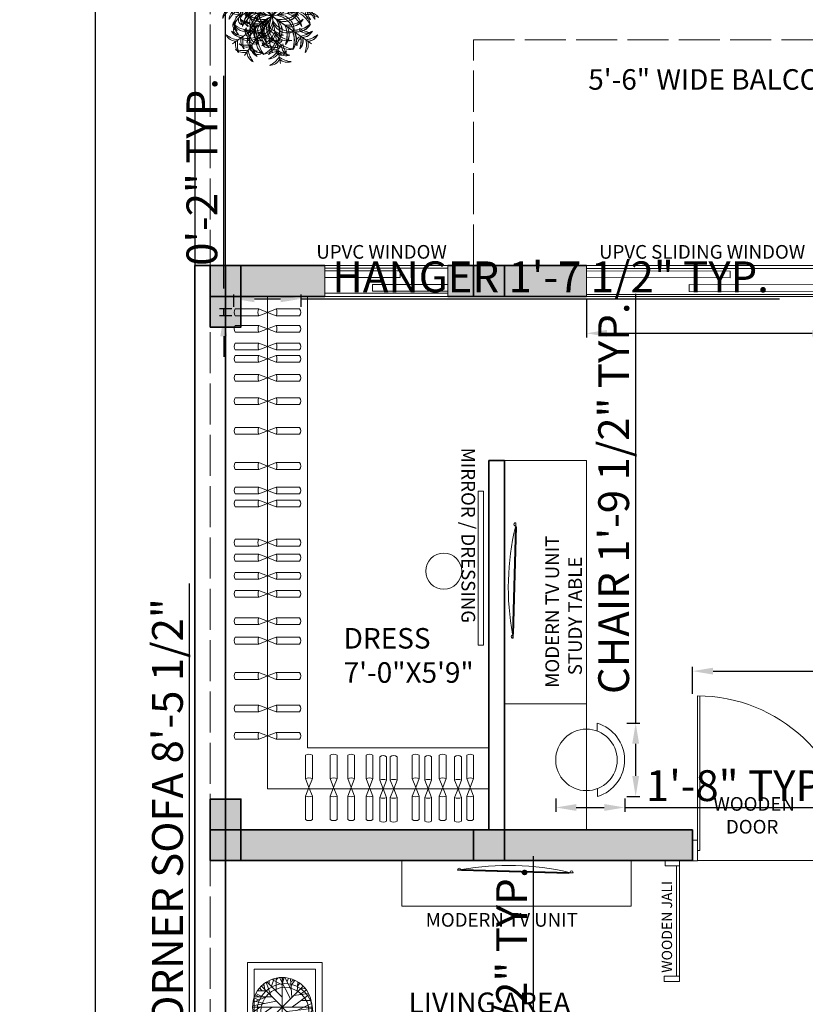
# Model space of a CAD drawing. Units: millimetres. Extents: x 595116 to 630915, y 909473 to 920225.
# Tile 122 of 134: x 629260 to 629490, y 919742 to 920030. Entities that reach past the tile are written whole.
import ezdxf

# ---------------------------------------------------------------- set-up
doc = ezdxf.new("R2010")
doc.units = ezdxf.units.MM
doc.linetypes.add('ACAD_ISO02W100', pattern=[15, 12, -3])
for name, color, linetype, lineweight in [('A-AREA-IDEN', 7, 'Continuous', 20), ('A-EQPM', 8, 'Continuous', 13), ('A-FLOR-OVHD', 253, 'ACAD_ISO02W100', 13), ('A-FLOR-SCRN', 31, 'Continuous', 18), ('A-FURN', 32, 'Continuous', 18), ('A-WALL', 1, 'Continuous', 35), ('A-WALL-PATT', 8, 'Continuous', 13), ('C-PROP', 7, 'Continuous', 25), ('C-PROP-REF', 240, 'ACAD_ISO02W100', 13), ('Column', 6, 'Continuous', 35), ('Dimension', 3, 'Continuous', 18), ('Doors', 31, 'Continuous', 20), ('L-PLNT', 85, 'Continuous', 13), ('Text', 7, 'Continuous', 18), ('Windows', 33, 'Continuous', 18)]:
    doc.layers.add(name, color=color, linetype=linetype, lineweight=lineweight)
doc.styles.get("Standard").update_dxf_attribs({"font": 'arial.ttf'})
doc.dimstyles.new('ISO-25', dxfattribs={"dimtxt": 9, "dimasz": 6, "dimexe": 1.25, "dimexo": 0.625, "dimtad": 1, "dimlunit": 4, "dimtxsty": 'Standard', "dimcen": 2.5, "dimadec": 0, "dimazin": 0, "dimtfac": 1, "dimtmove": 0, "dimatfit": 3, "dimfxl": 1, "dimarcsym": 0})

# ---------------------------------------------------------------- blocks, each defined once
blk = doc.blocks.new('KWD')
for points in [[(629753.63, 919957.93), (629752.54, 919957.93), (629752.54, 919953.43), (629753.63, 919953.43)], [(629787.45, 919957.93), (629787.45, 919953.43), (629788.54, 919953.43), (629788.54, 919957.93)]]:
    blk.add_lwpolyline(points, close=True)
blk.add_lwpolyline([(629753.63, 919921.79), (629753.63, 919955.68), (629754.13, 919955.68), (629754.13, 919921.8)])
blk.add_arc((629753.64, 919955.68), 33.88, 269.99, 356.196)
blk = doc.blocks.new('A$C5D061C3B')
for p, q in [((1.483, 6.082), (3.377, 3.377)), ((5.259, 6.086), (3.365, 3.381)), ((3.377, 6.679), (3.377, 3.377)), ((1.03, 5.716), (3.365, 3.381)), ((5.712, 5.712), (3.377, 3.377)), ((0.125, 3.951), (3.377, 3.377)), ((0.66, 1.487), (3.365, 3.381)), ((1.483, 0.672), (3.377, 3.377)), ((6.07, 1.487), (3.365, 3.381)), ((6.629, 3.951), (3.377, 3.377)), ((3.951, 0.125), (3.377, 3.377)), ((6.082, 1.483), (3.377, 3.377))]:
    blk.add_line(p, q)
for centre, radius, start, end in [((1.998, 5.617), 0.762, 125.37567, 188.71003), ((3.066, 5.423), 1.715, 151.62064, 180.92372), ((2.419, 5.816), 0.762, 115.37567, 178.71003), ((3.438, 5.44), 1.715, 141.62064, 170.92372), ((2.678, 5.447), 0.762, 115.37567, 178.71003), ((3.696, 5.07), 1.715, 141.62064, 170.92372), ((2.763, 5.924), 0.762, 36.28997, 99.62433), ((2.145, 5.032), 1.715, 44.07628, 73.37936), ((2.763, 5.474), 0.762, 36.28997, 99.62433), ((2.145, 4.581), 1.715, 44.07628, 73.37936), ((3.901, 5.939), 0.762, 125.37567, 188.71003), ((4.969, 5.745), 1.715, 151.62064, 180.92372), ((3.991, 5.924), 0.762, 80.37567, 143.71003), ((4.61, 5.032), 1.715, 106.62064, 135.92372), ((3.991, 5.474), 0.762, 80.37567, 143.71003), ((4.61, 4.581), 1.715, 106.62064, 135.92372), ((3.871, 5.832), 0.38, 94.742, 213.74753), ((4.447, 5.681), 0.826, 139.61802, 183.21064), ((4.064, 5.451), 0.762, 1.28997, 64.62433), ((3.046, 5.075), 1.715, 9.07628, 38.37936), ((3.305, 5.444), 1.715, 9.07628, 38.37936), ((4.323, 5.82), 0.762, 1.28997, 64.62433), ((4.744, 5.613), 0.762, 351.28997, 54.62433), ((3.676, 5.419), 1.715, 359.07628, 28.37936), ((1.13, 4.748), 0.762, 81.28997, 144.62433), ((1.324, 3.68), 1.715, 89.07628, 118.37936), ((1.413, 5.111), 0.762, 71.28997, 134.62433), ((1.419, 4.026), 1.715, 79.07628, 108.37936), ((1.671, 4.742), 0.762, 71.28997, 134.62433), ((2.317, 5.298), 0.762, 125.37567, 188.71003), ((1.991, 5.462), 0.38, 139.742, 258.74753), ((3.385, 5.104), 1.715, 151.62064, 180.92372), ((2.505, 5.763), 0.826, 184.61802, 228.21064), ((3.035, 5.062), 1.056, 129.60629, 199.75109), ((3.894, 4.989), 1.77, 149.96343, 193.62881), ((3.344, 5.089), 1.056, 119.60629, 189.75109), ((2.422, 4.799), 1.056, 25.24891, 95.39371), ((1.866, 4.14), 1.77, 31.37119, 75.03657), ((3.46, 4.637), 1.056, 129.60629, 199.75109), ((4.177, 4.869), 1.77, 139.96343, 183.62881), ((4.319, 4.565), 1.77, 149.96343, 193.62881), ((3.688, 4.597), 1.056, 119.60629, 189.75109), ((4.522, 4.377), 1.77, 139.96343, 183.62881), ((4.332, 4.799), 1.056, 84.60629, 154.75109), ((4.888, 4.14), 1.77, 104.96343, 148.62881), ((2.221, 4.381), 1.77, 356.37119, 40.03657), ((3.054, 4.602), 1.056, 350.24891, 60.39371), ((3.398, 5.094), 1.056, 350.24891, 60.39371), ((2.565, 4.873), 1.77, 356.37119, 40.03657), ((3.283, 4.633), 1.056, 340.24891, 50.39371), ((2.424, 4.56), 1.77, 346.37119, 30.03657), ((2.848, 4.985), 1.77, 346.37119, 30.03657), ((3.707, 5.058), 1.056, 340.24891, 50.39371), ((5.071, 4.746), 0.762, 45.37567, 108.71003), ((3.357, 5.1), 1.715, 359.07628, 28.37936), ((4.425, 5.294), 0.762, 351.28997, 54.62433), ((5.564, 4.807), 0.762, 80.37567, 143.71003), ((6.182, 3.914), 1.715, 106.62064, 135.92372), ((5.613, 4.744), 0.762, 35.37567, 98.71003), ((1.448, 4.43), 0.762, 81.28997, 144.62433), ((1.642, 3.362), 1.715, 89.07628, 118.37936), ((1.685, 3.712), 1.056, 70.24891, 140.39371), ((2.143, 4.564), 1.056, 164.60629, 234.75109), ((1.78, 3.994), 1.056, 60.24891, 130.39371), ((1.702, 3.136), 1.77, 66.37119, 110.03657), ((2.888, 4.998), 1.77, 184.96343, 228.62881), ((1.677, 3.657), 1.715, 79.07628, 108.37936), ((2.734, 4.46), 1.056, 164.60629, 234.75109), ((3.48, 4.893), 1.77, 184.96343, 228.62881), ((3.25, 4.435), 1.029, 156.36542, 256.57406), ((3.862, 4.761), 1.557, 176.81221, 238.33354), ((2.422, 4.198), 1.056, 25.24891, 95.39371), ((1.866, 3.54), 1.77, 31.37119, 75.03657), ((3.868, 4.321), 1.029, 121.36542, 221.57406), ((4.556, 4.237), 1.557, 141.81221, 203.33354), ((4.035, 4.215), 1.029, 111.36542, 211.57406), ((2.707, 4.219), 1.029, 328.42594, 68.63458), ((2.044, 4.017), 1.557, 346.66646, 48.18779), ((4.698, 4.013), 1.557, 131.81221, 193.33354), ((4.332, 4.198), 1.056, 84.60629, 154.75109), ((4.888, 3.54), 1.77, 104.96343, 148.62881), ((2.187, 4.233), 1.557, 336.66646, 38.18779), ((2.875, 4.316), 1.029, 318.42594, 58.63458), ((2.893, 4.761), 1.557, 301.66646, 3.18779), ((3.504, 4.435), 1.029, 283.42594, 23.63458), ((5.04, 3.14), 1.77, 69.96343, 113.62881), ((4.963, 3.998), 1.056, 49.60629, 119.75109), ((3.275, 4.893), 1.77, 311.37119, 355.03657), ((4.02, 4.46), 1.056, 305.24891, 15.39371), ((5.058, 3.707), 1.056, 39.60629, 109.75109), ((5.065, 3.661), 1.715, 71.62064, 100.92372), ((3.866, 4.998), 1.77, 311.37119, 355.03657), ((5.1, 3.357), 1.715, 61.62064, 90.92372), ((5.294, 4.425), 0.762, 35.37567, 98.71003), ((4.611, 4.564), 1.056, 305.24891, 15.39371), ((5.419, 3.676), 1.715, 61.62064, 90.92372), ((0.975, 4.424), 0.762, 160.37567, 223.71003), ((1.962, 4.878), 1.715, 186.62064, 215.92372), ((1.419, 4.346), 0.762, 160.37567, 223.71003), ((2.405, 4.8), 1.715, 186.62064, 215.92372), ((1.12, 4.31), 0.38, 94.742, 213.74753), ((1.696, 4.159), 0.826, 139.61802, 183.21064), ((1.757, 2.853), 1.77, 76.37119, 120.03657), ((1.588, 3.666), 0.38, 94.742, 213.74753), ((2.109, 3.287), 1.056, 70.24891, 140.39371), ((2.182, 2.428), 1.77, 76.37119, 120.03657), ((2.165, 3.515), 0.826, 139.61802, 183.21064), ((2.124, 3.502), 1.056, 60.24891, 130.39371), ((2.046, 2.644), 1.77, 66.37119, 110.03657), ((2.365, 3.045), 1.029, 38.42594, 138.63458), ((2.387, 3.752), 0.574, 99.98654, 199.40339), ((3.599, 3.314), 1.651, 142.57587, 170.89417), ((2.358, 3.686), 1.029, 3.42594, 103.63458), ((1.93, 3.14), 1.557, 21.66646, 83.18779), ((2.84, 3.739), 0.372, 69.22575, 210.12788), ((3.109, 3.59), 0.515, 105.43977, 183.66943), ((4.397, 3.686), 1.029, 76.36542, 176.57406), ((4.824, 3.14), 1.557, 96.81221, 158.33354), ((4.377, 3.05), 1.029, 41.36542, 141.57406), ((4.696, 2.648), 1.77, 69.96343, 113.62881), ((4.618, 3.506), 1.056, 49.60629, 119.75109), ((4.56, 2.424), 1.77, 59.96343, 103.62881), ((4.633, 3.283), 1.056, 39.60629, 109.75109), ((4.985, 2.848), 1.77, 59.96343, 103.62881), ((4.988, 5.812), 1.715, 279.07628, 308.37936), ((5.365, 4.794), 0.762, 271.28997, 334.62433), ((4.349, 4.8), 1.715, 324.07628, 353.37936), ((5.335, 4.346), 0.762, 316.28997, 19.62433), ((4.793, 4.878), 1.715, 324.07628, 353.37936), ((5.779, 4.424), 0.762, 316.28997, 19.62433), ((0.762, 3.214), 0.762, 116.28997, 179.62433), ((1.534, 2.451), 1.715, 124.07628, 153.37936), ((1.206, 3.136), 0.762, 116.28997, 179.62433), ((1.977, 2.373), 1.715, 124.07628, 153.37936), ((1.062, 4.452), 0.826, 229.61802, 273.21064), ((0.91, 3.875), 0.38, 184.742, 303.74753), ((1.811, 2.684), 1.056, 105.24891, 175.39371), ((2.363, 2.022), 1.77, 111.37119, 155.03657), ((2.185, 0.015), 3.567, 70.47721, 111.6585), ((1.447, 3.129), 0.376, 122.05775, 257.85325), ((1.751, 3.126), 0.529, 140.18449, 223.65396), ((2.403, 2.58), 1.056, 105.24891, 175.39371), ((2.955, 1.917), 1.77, 111.37119, 155.03657), ((2.007, 3.071), 0.506, 93.87442, 233.97626), ((2.426, 2.879), 1.029, 48.42594, 148.63458), ((2.51, 2.191), 1.557, 66.66646, 128.18779), ((2.729, 4.702), 1.557, 221.81221, 283.33354), ((2.527, 4.039), 1.029, 201.36542, 301.57406), ((2.328, 2.353), 1.557, 56.66646, 118.18779), ((4.912, 0.157), 3.567, 115.47721, 156.6585), ((2.489, 2.932), 0.825, 128.75364, 199.09705), ((2.896, 2.427), 1.029, 83.42594, 183.63458), ((3.359, 1.911), 1.557, 101.66646, 163.18779), ((2.903, 2.8), 0.855, 116.44767, 194.36723), ((4.744, 1.779), 2.789, 140.40074, 163.13904), ((2.741, 3.253), 0.372, 114.22575, 255.12788), ((3.037, 3.338), 0.515, 150.43977, 228.66943), ((6.727, 2.189), 3.567, 160.47721, 201.6585), ((4.414, 2.358), 1.557, 61.81221, 123.33354), ((4.233, 2.187), 1.557, 51.81221, 113.33354), ((4.316, 2.875), 1.029, 31.36542, 131.57406), ((4.001, 4.702), 1.557, 256.66646, 318.18779), ((4.013, 4.698), 1.557, 256.66646, 318.18779), ((4.203, 4.039), 1.029, 238.42594, 338.63458), ((4.215, 4.035), 1.029, 238.42594, 338.63458), ((3.395, 1.911), 1.557, 16.81221, 78.33354), ((3.858, 2.427), 1.029, 356.36542, 96.57406), ((3.799, 1.917), 1.77, 24.96343, 68.62881), ((4.352, 2.58), 1.056, 4.60629, 74.75109), ((4.391, 2.022), 1.77, 24.96343, 68.62881), ((4.943, 2.684), 1.056, 4.60629, 74.75109), ((6.053, 3.533), 0.38, 146.25247, 265.258), ((5.741, 1.774), 1.715, 61.62064, 90.92372), ((4.777, 2.373), 1.715, 26.62064, 55.92372), ((6.629, 3.684), 0.826, 176.78936, 220.38198), ((5.935, 2.842), 0.762, 35.37567, 98.71003), ((5.549, 3.136), 0.762, 0.37567, 63.71003), ((1.067, 2.749), 0.376, 122.05775, 257.85325), ((1.873, 4.181), 1.77, 229.96343, 273.62881), ((1.653, 3.348), 1.056, 209.60629, 279.75109), ((1.37, 2.745), 0.529, 140.18449, 223.65396), ((2.145, 3.693), 1.056, 209.60629, 279.75109), ((2.365, 4.526), 1.77, 229.96343, 273.62881), ((2.328, 4.401), 1.557, 241.81221, 303.33354), ((2.365, 3.709), 1.029, 221.36542, 321.57406), ((2.412, 2.943), 0.574, 144.98654, 244.40339), ((3.578, 3.49), 1.651, 187.57587, 215.89417), ((4.099, 2.051), 1.77, 156.37119, 200.03657), ((1.911, 3.359), 1.557, 286.81221, 348.33354), ((2.427, 2.896), 1.029, 266.36542, 6.57406), ((3.45, 2.634), 0.855, 161.44767, 239.36723), ((3.003, 2.844), 0.372, 159.22575, 300.12788), ((3.152, 3.113), 0.515, 195.43977, 273.66943), ((3.697, 2.369), 1.029, 128.42594, 228.63458), ((5.474, 3.214), 2.789, 185.40074, 208.13904), ((4.389, 2.332), 1.557, 146.66646, 208.18779), ((4.035, 2.539), 1.029, 148.42594, 248.63458), ((4.698, 2.741), 1.557, 166.66646, 228.18779), ((4.435, 3.25), 1.029, 193.42594, 293.63458), ((4.761, 3.862), 1.557, 211.66646, 273.18779), ((2.341, 2.332), 1.557, 331.81221, 33.33354), ((2.353, 2.328), 1.557, 331.81221, 33.33354), ((3.033, 2.369), 1.029, 311.36542, 51.57406), ((3.045, 2.365), 1.029, 311.36542, 51.57406), ((4.365, 4.526), 1.77, 266.37119, 310.03657), ((2.632, 2.051), 1.77, 339.96343, 23.62881), ((4.377, 4.522), 1.77, 266.37119, 310.03657), ((2.644, 2.046), 1.77, 339.96343, 23.62881), ((4.585, 3.693), 1.056, 260.24891, 330.39371), ((4.597, 3.688), 1.056, 260.24891, 330.39371), ((4.857, 4.181), 1.77, 266.37119, 310.03657), ((4.869, 4.177), 1.77, 266.37119, 310.03657), ((5.077, 3.348), 1.056, 260.24891, 330.39371), ((5.089, 3.344), 1.056, 260.24891, 330.39371), ((0.926, 2.424), 0.762, 205.37567, 268.71003), ((1.303, 3.442), 1.715, 231.62064, 260.92372), ((1.672, 3.7), 1.715, 231.62064, 260.92372), ((1.295, 2.682), 0.762, 205.37567, 268.71003), ((1.122, 2.441), 0.38, 139.742, 258.74753), ((1.636, 2.741), 0.826, 184.61802, 228.21064), ((2.046, 4.111), 1.77, 249.96343, 293.62881), ((2.124, 3.252), 1.056, 229.60629, 299.75109), ((1.908, 2.317), 0.38, 139.742, 258.74753), ((2.422, 2.617), 0.826, 184.61802, 228.21064), ((2.748, 1.784), 1.056, 150.24891, 220.39371), ((3.607, 1.706), 1.77, 156.37119, 200.03657), ((2.624, 2.192), 0.506, 138.87442, 278.97626), ((3.24, 2.128), 1.056, 150.24891, 220.39371), ((3.064, 2.435), 0.825, 173.75364, 244.09705), ((3.428, 3.603), 1.651, 232.57587, 260.89417), ((2.99, 2.391), 0.574, 189.98654, 289.40339), ((3.688, 2.157), 1.056, 170.24891, 240.39371), ((1.917, 2.955), 1.77, 294.96343, 338.62881), ((2.58, 2.403), 1.056, 274.60629, 344.75109), ((4.522, 2.378), 1.77, 176.37119, 220.03657), ((3.942, 2.908), 0.855, 206.44767, 284.36723), ((4.963, 4.749), 2.789, 230.40074, 253.13904), ((4.893, 3.48), 1.77, 221.37119, 265.03657), ((4.46, 2.734), 1.056, 215.24891, 285.39371), ((3.49, 2.128), 1.056, 319.60629, 29.75109), ((3.502, 2.124), 1.056, 319.60629, 29.75109), ((3.124, 1.706), 1.77, 339.96343, 23.62881), ((3.136, 1.702), 1.77, 339.96343, 23.62881), ((3.982, 1.784), 1.056, 319.60629, 29.75109), ((3.994, 1.78), 1.056, 319.60629, 29.75109), ((6.244, 3.948), 1.715, 234.07628, 263.37936), ((5.79, 2.962), 0.762, 226.28997, 289.62433), ((5.058, 3.7), 1.715, 279.07628, 308.37936), ((5.07, 3.696), 1.715, 279.07628, 308.37936), ((5.435, 2.682), 0.762, 271.28997, 334.62433), ((5.447, 2.678), 0.762, 271.28997, 334.62433), ((5.427, 3.442), 1.715, 279.07628, 308.37936), ((5.44, 3.438), 1.715, 279.07628, 308.37936), ((5.804, 2.424), 0.762, 271.28997, 334.62433), ((5.816, 2.419), 0.762, 271.28997, 334.62433), ((1.631, 1.417), 0.762, 161.28997, 224.62433), ((2.717, 1.423), 1.715, 169.07628, 198.37936), ((1.702, 3.619), 1.77, 249.96343, 293.62881), ((1.78, 2.76), 1.056, 229.60629, 299.75109), ((1.671, 2.012), 0.762, 225.37567, 288.71003), ((1.677, 3.098), 1.715, 251.62064, 280.92372), ((2, 1.676), 0.762, 161.28997, 224.62433), ((3.086, 1.681), 1.715, 169.07628, 198.37936), ((2.188, 1.837), 0.376, 167.05775, 302.85325), ((2.188, 1.299), 0.376, 167.05775, 302.85325), ((2.405, 2.049), 0.529, 185.18449, 268.65396), ((2.405, 1.511), 0.529, 185.18449, 268.65396), ((3.696, 1.684), 1.715, 189.07628, 218.37936), ((3.344, 1.665), 1.056, 170.24891, 240.39371), ((4.177, 1.886), 1.77, 176.37119, 220.03657), ((3.227, 2.169), 0.826, 229.61802, 273.21064), ((3.076, 1.593), 0.38, 184.742, 303.74753), ((2.022, 2.363), 1.77, 294.96343, 338.62881), ((2.684, 1.811), 1.056, 274.60629, 344.75109), ((3.81, 2.493), 0.825, 218.75364, 289.09705), ((3.671, 2.011), 0.506, 183.87442, 323.97626), ((3.616, 1.755), 0.529, 230.18449, 313.65396), ((3.613, 1.452), 0.376, 212.05775, 347.85325), ((4.998, 2.888), 1.77, 221.37119, 265.03657), ((4.564, 2.143), 1.056, 215.24891, 285.39371), ((4.79, 1.377), 0.762, 181.28997, 244.62433), ((5.808, 1.754), 1.715, 189.07628, 218.37936), ((5.385, 1.584), 0.38, 101.25247, 220.258), ((5.899, 1.283), 0.826, 131.78936, 175.38198), ((3.645, 1.681), 1.715, 341.62064, 10.92372), ((4.73, 1.676), 0.762, 315.37567, 18.71003), ((3.657, 1.677), 1.715, 341.62064, 10.92372), ((4.742, 1.671), 0.762, 315.37567, 18.71003), ((4.014, 1.423), 1.715, 341.62064, 10.92372), ((5.099, 1.417), 0.762, 315.37567, 18.71003), ((1.419, 2.729), 1.715, 251.62064, 280.92372), ((1.413, 1.643), 0.762, 225.37567, 288.71003), ((2.419, 0.938), 0.762, 181.28997, 244.62433), ((3.438, 1.315), 1.715, 189.07628, 218.37936), ((2.678, 1.307), 0.762, 181.28997, 244.62433), ((2.583, 1.701), 0.826, 229.61802, 273.21064), ((2.432, 1.124), 0.38, 184.742, 303.74753), ((2.373, 1.977), 1.715, 296.62064, 325.92372), ((3.136, 1.206), 0.762, 270.37567, 333.71003), ((3.68, 0.113), 0.826, 86.78936, 130.38198), ((3.528, 0.69), 0.38, 56.25247, 175.258), ((3.997, 1.374), 0.529, 230.18449, 313.65396), ((3.994, 1.071), 0.376, 212.05775, 347.85325), ((4.8, 2.405), 1.715, 234.07628, 263.37936), ((4.346, 1.419), 0.762, 226.28997, 289.62433), ((2.451, 1.534), 1.715, 296.62064, 325.92372), ((3.214, 0.762), 0.762, 270.37567, 333.71003), ((4.878, 1.962), 1.715, 234.07628, 263.37936), ((4.424, 0.975), 0.762, 226.28997, 289.62433)]:
    blk.add_arc(centre, radius, start, end)
blk = doc.blocks.new('*D128')
at = {"layer": 'Defpoints', "color": 0, "transparency": 16777216}
for p in [(629311.54, 920089.43), (629282.4, 919141.93), (629311.54, 919141.93)]:
    blk.add_point(p, dxfattribs=at)
at = {"layer": 'Dimension', "color": 0, "lineweight": -2, "transparency": 16777216}
for p, q in [((629310.92, 920089.43), (629281.15, 920089.43)), ((629282.4, 920083.43), (629282.4, 919147.93)), ((629310.92, 919141.93), (629281.15, 919141.93))]:
    blk.add_line(p, q, dxfattribs=at)
at = {"layer": 'Dimension', "color": 0, "transparency": 16777216}
for points in [[(629281.4, 920083.43), (629283.4, 920083.43), (629282.4, 920089.43)], [(629281.4, 919147.93), (629283.4, 919147.93), (629282.4, 919141.93)]]:
    blk.add_solid(points, dxfattribs=at)
at = {"layer": 'Dimension', "color": 0, "transparency": 16777216, "insert": (629271.16, 919615.68), "char_height": 9, "attachment_point": 5, "rotation": 90}
blk.add_mtext('78\'-11{\\H1x;\\S1/2;}"', dxfattribs=at)
blk = doc.blocks.new('TV-PLAN')
for p, q in [((2.04, 32.58), (1.21, 1.19)), ((2.14, 32.58), (1.31, 1.19)), ((2.24, 32.58), (1.41, 1.19)), ((2.34, 32.57), (1.51, 1.18)), ((2.04, 32.58), (2.34, 32.57)), ((2.14, 32.58), (2.14, 33.76)), ((2.19, 32.58), (2.19, 33.76)), ((1.21, 1.19), (1.51, 1.18)), ((1.31, 1.19), (1.31, 0.01)), ((1.36, 1.19), (1.36, 0.01))]:
    blk.add_line(p, q)
for centre, radius, start, end in [((76.63, 14.9), 76.65, 166.662, 190.3006), ((2.09, 33.31), 0.462, 77.1755, 282.8245), ((1.26, 0.46), 0.462, 77.1755, 282.8245)]:
    blk.add_arc(centre, radius, start, end)
blk = doc.blocks.new('WARDROBE-HANGER')
for p, q in [((9.73, 1), (9.73, 1)), ((9.73, 1), (12.27, 0)), ((9.73, 1), (9.73, 1)), ((12.27, 2), (19.15, 2)), ((0.32, 0), (7.19, 0)), ((12.27, 0), (19.15, 0))]:
    blk.add_line(p, q)
for points in [[(7.19, 2), (0.32, 2, 0.315389), (0.32, 0)], [(9.73, 1), (7.19, 2, 0.225748), (7.19, 0), (9.73, 1), (12.27, 2)]]:
    blk.add_lwpolyline(points, format="xyb")
for centre, radius, start, end in [((10.17, 1), 2.33, 334.5576, 25.4424), ((17.71, 1), 1.74, 324.9906, 35.0094)]:
    blk.add_arc(centre, radius, start, end)
blk = doc.blocks.new('PLANTER-RECT')
for p, q in [((6.36, 22.38), (6.39, 23.42)), ((7, 21.72), (7.79, 23.98)), ((7.12, 23.71), (10.18, 22.15)), ((8.37, 23.58), (9.03, 24.24)), ((8.4, 20.29), (8.37, 24.14)), ((9.42, 24.27), (12.57, 18.07)), ((10.54, 23.58), (9.98, 24.3)), ((10.18, 24.32), (10.18, 6.97)), ((10.26, 22.67), (10.71, 24.27)), ((12.83, 20.78), (10.97, 24.27)), ((11.6, 23.09), (12.04, 24.11)), ((13.03, 18.46), (12.55, 23.98)), ((12.65, 23.03), (13.54, 23.62)), ((12.75, 21.95), (13.87, 23.49)), ((2.98, 20.39), (5.45, 20.39)), ((3.56, 21.17), (4.33, 20.42)), ((3.84, 20.91), (3.77, 21.46)), ((16.26, 21.71), (4.11, 9.57)), ((16.26, 9.57), (4.11, 21.71)), ((4.38, 22.08), (4.91, 21.89)), ((4.83, 22.44), (5.09, 20.78)), ((5.47, 22.93), (6.82, 19.05)), ((5.67, 23.03), (10.15, 18.56)), ((14.76, 23), (14.56, 20.06)), ((14.68, 21.79), (15.37, 22.61)), ((15.42, 19.28), (17.25, 20.71)), ((15.55, 21.01), (16.92, 21.07)), ((1.55, 16.05), (8.45, 17.38)), ((5.52, 18.62), (1.63, 16.99)), ((1.7, 17.48), (4.99, 16.73)), ((1.93, 18.23), (3.38, 17.78)), ((2.09, 18.66), (7.18, 18.66)), ((2.26, 19.18), (3.28, 18.69)), ((2.49, 19.6), (4.38, 18.66)), ((18.04, 19.31), (13.21, 15.69)), ((13.56, 19.02), (17.89, 19.6)), ((15.75, 17.58), (18.6, 17.61)), ((1.51, 15.64), (18.86, 15.64)), ((1.55, 14.94), (2.34, 14.68)), ((3.64, 15.62), (1.65, 14.19)), ((2.29, 12.07), (7.25, 15.66)), ((11.53, 14.32), (18.81, 15.23)), ((14.43, 14.68), (18.78, 16.67)), ((1.73, 13.86), (4.91, 13.96)), ((1.93, 12.98), (3.64, 13.05)), ((2.57, 13.01), (2.16, 12.46)), ((2.49, 11.67), (7.76, 13.24)), ((3.36, 12.85), (2.93, 11.84)), ((4.99, 12.39), (3.82, 9.78)), ((7.3, 12.72), (6.06, 8.02)), ((8.04, 13.47), (8.07, 7.3)), ((8.73, 14.19), (9.82, 7.01)), ((10.18, 12.88), (13.92, 7.86)), ((12.88, 12.95), (14.05, 7.92)), ((12.9, 12.95), (18.48, 13.14)), ((14, 12.98), (18.71, 14.22)), ((15.7, 13.01), (17.76, 11.45)), ((16.82, 12.16), (18.22, 12.43)), ((4.55, 11.45), (2.75, 11.22)), ((3.46, 11.28), (3.03, 10.79)), ((5.5, 10.96), (3.23, 10.5)), ((3.87, 10.63), (3.43, 10.24)), ((6.62, 10.17), (4.58, 9.03)), ((6.39, 9.29), (5.17, 8.61)), ((8.07, 10.4), (6.18, 7.99)), ((8.07, 8.8), (6.57, 7.79)), ((7.07, 9.06), (7.3, 7.53)), ((8.07, 10.99), (9.62, 7.04)), ((8.96, 8.77), (8.52, 7.17)), ((9.29, 10.4), (12.78, 7.4)), ((11.04, 8.9), (11.71, 7.17)), ((13.49, 10.37), (15.29, 8.64)), ((13.77, 9.16), (13.51, 7.69)), ((14.58, 11.28), (14.86, 8.41)), ((14.73, 11.12), (17.36, 10.83)), ((16.19, 10.92), (16.85, 10.14)), ((9.26, 8.02), (8.83, 7.14)), ((11.4, 7.96), (10.74, 7.04))]:
    blk.add_line(p, q)
for points in [[(0, 28.69), (21.89, 28.69), (21.89, 0), (0, 0)], [(2, 26.69), (19.89, 26.69), (19.89, 2), (2, 2)]]:
    blk.add_lwpolyline(points, close=True)
for centre, radius in [((10.18, 15.64), 8.67), ((10.95, 14.35), 8.14), ((10.95, 14.35), 7.03)]:
    blk.add_circle(centre, radius)
blk = doc.blocks.new('WIN-UPVC-3FT')
for p, q in [((0, 0), (0, 9)), ((0, 9), (36, 9)), ((36, 0), (36, 9)), ((0, 7.5), (22, 7.5)), ((22, 7.5), (22, 5.5)), ((0, 5.5), (22, 5.5)), ((14, 3.5), (36, 3.5)), ((14, 3.5), (14, 1.5)), ((14, 1.5), (36, 1.5)), ((0, 0), (36, 0))]:
    blk.add_line(p, q)
blk.add_lwpolyline([(0, 8.25), (36, 8.25), (36, 0.89), (0, 0.89)], close=True)
blk = doc.blocks.new('WIN-SLIDING-6FT')
for p, q in [((0, 0), (0, 9)), ((0, 9), (72, 9)), ((72, 0), (72, 9)), ((0.01, 7.5), (42, 7.41)), ((42, 7.41), (42, 5.41)), ((0, 5.5), (42, 5.41)), ((30, 3.44), (72, 3.35)), ((30, 3.44), (30, 1.44)), ((30, 1.44), (71.99, 1.35)), ((0, 0), (72, 0))]:
    blk.add_line(p, q)
blk.add_lwpolyline([(0, 8.12), (72, 8.12), (72, 0.59), (0, 0.59)], close=True)
blk = doc.blocks.new('CHAIR-ROUND')
for p, q in [((12.11, 21.41), (12.12, 19.12)), ((12.2, 2.29), (12.22, 0))]:
    blk.add_line(p, q)
blk.add_circle((8.99, 10.69), 8.99)
blk.add_arc((8.99, 10.69), 11.16, 286.7943, 73.7898)
blk = doc.blocks.new('COLUMN-SQUARE-9IN')
h = blk.add_hatch(color=256)
h.dxf.hatch_style = 1
h.paths.add_polyline_path([(9, 9), (0, 9), (0, 0), (9, 0)])
blk.add_lwpolyline([(0, 9), (9, 9), (9, 0), (0, 0)], close=True)
blk = doc.blocks.new('COLUMN-RECT-9X18')
h = blk.add_hatch(color=256)
h.dxf.hatch_style = 1
h.paths.add_polyline_path([(9, 18), (0, 18), (0, 0), (9, 0)])
blk.add_lwpolyline([(0, 18), (9, 18), (9, 0), (0, 0)], close=True)
blk = doc.blocks.new('*D158')
at = {"layer": 'Defpoints', "color": 0, "transparency": 16777216}
for p in [(629342.62, 919948.21), (629322.95, 919945.26), (629342.62, 919945.26)]:
    blk.add_point(p, dxfattribs=at)
at = {"layer": 'Dimension', "color": 0, "lineweight": -2, "transparency": 16777216}
for p, q in [((629322.95, 919945.88), (629322.95, 919949.46)), ((629328.95, 919948.21), (629336.62, 919948.21)), ((629342.62, 919945.88), (629342.62, 919949.46)), ((629342.62, 919948.21), (629482.5, 919948.21))]:
    blk.add_line(p, q, dxfattribs=at)
at = {"layer": 'Dimension', "color": 0, "transparency": 16777216}
for points in [[(629328.95, 919949.21), (629328.95, 919947.21), (629322.95, 919948.21)], [(629336.62, 919949.21), (629336.62, 919947.21), (629342.62, 919948.21)]]:
    blk.add_solid(points, dxfattribs=at)
at = {"layer": 'Dimension', "color": 0, "transparency": 16777216, "insert": (629415.56, 919953.48), "char_height": 9, "attachment_point": 5}
blk.add_mtext('HANGER 1\'-7 1/2" TYP.', dxfattribs=at)
blk = doc.blocks.new('*D159')
at = {"layer": 'Defpoints', "color": 0, "transparency": 16777216}
for p in [(629320, 919945.26), (629322.95, 919945.26), (629322.95, 919943.26)]:
    blk.add_point(p, dxfattribs=at)
at = {"layer": 'Dimension', "color": 0, "lineweight": -2, "transparency": 16777216}
for p, q in [((629320, 919951.26), (629320, 920013.37)), ((629322.33, 919945.26), (629318.75, 919945.26)), ((629320, 919943.26), (629320, 919945.26)), ((629322.33, 919943.26), (629318.75, 919943.26)), ((629320, 919937.26), (629320, 919931.26))]:
    blk.add_line(p, q, dxfattribs=at)
at = {"layer": 'Dimension', "color": 0, "transparency": 16777216}
for points in [[(629319, 919951.26), (629321, 919951.26), (629320, 919945.26)], [(629319, 919937.26), (629321, 919937.26), (629320, 919943.26)]]:
    blk.add_solid(points, dxfattribs=at)
at = {"layer": 'Dimension', "color": 0, "transparency": 16777216, "insert": (629314.78, 919985.31), "char_height": 9, "attachment_point": 5, "rotation": 90}
blk.add_mtext('0\'-2" TYP.', dxfattribs=at)
blk = doc.blocks.new('*D162')
at = {"layer": 'Defpoints', "color": 0, "transparency": 16777216}
for p in [(629505.04, 919832.11), (629505.04, 919783.93), (629512.27, 919783.93)]:
    blk.add_point(p, dxfattribs=at)
at = {"layer": 'Dimension', "color": 0, "lineweight": -2, "transparency": 16777216}
for p, q in [((629505.67, 919832.11), (629513.52, 919832.11)), ((629512.27, 919826.11), (629512.27, 919789.93)), ((629505.67, 919783.93), (629513.52, 919783.93)), ((629512.27, 919783.93), (629512.27, 919681.05))]:
    blk.add_line(p, q, dxfattribs=at)
at = {"layer": 'Dimension', "color": 0, "transparency": 16777216}
for points in [[(629511.27, 919826.11), (629513.27, 919826.11), (629512.27, 919832.11)], [(629511.27, 919789.93), (629513.27, 919789.93), (629512.27, 919783.93)]]:
    blk.add_solid(points, dxfattribs=at)
at = {"layer": 'Dimension', "color": 0, "transparency": 16777216, "insert": (629506.99, 919729.49), "char_height": 9, "attachment_point": 5, "rotation": 90}
blk.add_mtext('DOOR 4\'-0" TYP.', dxfattribs=at)
blk = doc.blocks.new('*D163')
at = {"layer": 'Defpoints', "color": 0, "transparency": 16777216}
for p in [(629505.04, 919839.34), (629457.04, 919832.11), (629505.04, 919832.11)]:
    blk.add_point(p, dxfattribs=at)
at = {"layer": 'Dimension', "color": 0, "lineweight": -2, "transparency": 16777216}
for p, q in [((629457.04, 919832.74), (629457.04, 919840.59)), ((629463.04, 919839.34), (629499.04, 919839.34)), ((629505.04, 919832.74), (629505.04, 919840.59)), ((629505.04, 919839.34), (629567.51, 919839.34))]:
    blk.add_line(p, q, dxfattribs=at)
at = {"layer": 'Dimension', "color": 0, "transparency": 16777216}
for points in [[(629463.04, 919840.34), (629463.04, 919838.34), (629457.04, 919839.34)], [(629499.04, 919840.34), (629499.04, 919838.34), (629505.04, 919839.34)]]:
    blk.add_solid(points, dxfattribs=at)
at = {"layer": 'Dimension', "color": 0, "transparency": 16777216, "insert": (629539.28, 919844.56), "char_height": 9, "attachment_point": 5}
blk.add_mtext('4\'-0" TYP.', dxfattribs=at)
blk = doc.blocks.new('*D178')
at = {"layer": 'Defpoints', "color": 0, "transparency": 16777216}
for p in [(629437.23, 919824.11), (629440.44, 919824.11), (629437.23, 919802.7)]:
    blk.add_point(p, dxfattribs=at)
at = {"layer": 'Dimension', "color": 0, "lineweight": -2, "transparency": 16777216}
for p, q in [((629440.44, 919824.11), (629440.44, 919949.69)), ((629437.86, 919824.11), (629441.69, 919824.11)), ((629440.44, 919808.7), (629440.44, 919818.11)), ((629437.86, 919802.7), (629441.69, 919802.7))]:
    blk.add_line(p, q, dxfattribs=at)
at = {"layer": 'Dimension', "color": 0, "transparency": 16777216}
for points in [[(629439.44, 919818.11), (629441.44, 919818.11), (629440.44, 919824.11)], [(629439.44, 919808.7), (629441.44, 919808.7), (629440.44, 919802.7)]]:
    blk.add_solid(points, dxfattribs=at)
at = {"layer": 'Dimension', "color": 0, "transparency": 16777216, "insert": (629435.16, 919889.9), "char_height": 9, "attachment_point": 5, "rotation": 90}
blk.add_mtext('CHAIR 1\'-9 1/2" TYP.', dxfattribs=at)
blk = doc.blocks.new('*D179')
at = {"layer": 'Defpoints', "color": 0, "transparency": 16777216}
for p in [(629417.05, 919802.7), (629437.23, 919802.7), (629437.23, 919799.48)]:
    blk.add_point(p, dxfattribs=at)
at = {"layer": 'Dimension', "color": 0, "lineweight": -2, "transparency": 16777216}
for p, q in [((629417.05, 919802.07), (629417.05, 919798.23)), ((629437.23, 919802.07), (629437.23, 919798.23)), ((629423.05, 919799.48), (629431.23, 919799.48)), ((629437.23, 919799.48), (629498.49, 919799.48))]:
    blk.add_line(p, q, dxfattribs=at)
at = {"layer": 'Dimension', "color": 0, "transparency": 16777216}
for points in [[(629423.05, 919800.48), (629423.05, 919798.48), (629417.05, 919799.48)], [(629431.23, 919800.48), (629431.23, 919798.48), (629437.23, 919799.48)]]:
    blk.add_solid(points, dxfattribs=at)
at = {"layer": 'Dimension', "color": 0, "transparency": 16777216, "insert": (629470.86, 919804.7), "char_height": 9, "attachment_point": 5}
blk.add_mtext('1\'-8" TYP.', dxfattribs=at)
blk = doc.blocks.new('*D188')
at = {"layer": 'Defpoints', "color": 0, "transparency": 16777216}
for p in [(629410.6, 919641.11), (629414.9, 919641.11), (629414.9, 919612.42)]:
    blk.add_point(p, dxfattribs=at)
at = {"layer": 'Dimension', "color": 0, "lineweight": -2, "transparency": 16777216}
for p, q in [((629410.6, 919641.11), (629410.6, 919785.23)), ((629414.27, 919641.11), (629409.35, 919641.11)), ((629410.6, 919618.42), (629410.6, 919635.11)), ((629414.27, 919612.42), (629409.35, 919612.42))]:
    blk.add_line(p, q, dxfattribs=at)
at = {"layer": 'Dimension', "color": 0, "transparency": 16777216}
for points in [[(629409.6, 919635.11), (629411.6, 919635.11), (629410.6, 919641.11)], [(629409.6, 919618.42), (629411.6, 919618.42), (629410.6, 919612.42)]]:
    blk.add_solid(points, dxfattribs=at)
at = {"layer": 'Dimension', "color": 0, "transparency": 16777216, "insert": (629405.32, 919716.17), "char_height": 9, "attachment_point": 5, "rotation": 90}
blk.add_mtext('PLANTER 2\'-4 1/2" TYP.', dxfattribs=at)
blk = doc.blocks.new('*D192')
at = {"layer": 'Defpoints', "color": 0, "transparency": 16777216}
for p in [(629426.04, 919948.93), (629498.04, 919948.93), (629498.04, 919938.13)]:
    blk.add_point(p, dxfattribs=at)
at = {"layer": 'Dimension', "color": 0, "lineweight": -2, "transparency": 16777216}
for p, q in [((629426.04, 919948.3), (629426.04, 919936.88)), ((629498.04, 919948.3), (629498.04, 919936.88)), ((629432.04, 919938.13), (629492.04, 919938.13)), ((629498.04, 919938.13), (629672.56, 919938.13))]:
    blk.add_line(p, q, dxfattribs=at)
at = {"layer": 'Dimension', "color": 0, "transparency": 16777216}
for points in [[(629432.04, 919939.13), (629432.04, 919937.13), (629426.04, 919938.13)], [(629492.04, 919939.13), (629492.04, 919937.13), (629498.04, 919938.13)]]:
    blk.add_solid(points, dxfattribs=at)
at = {"layer": 'Dimension', "color": 0, "transparency": 16777216, "insert": (629588.3, 919943.41), "char_height": 9, "attachment_point": 5}
blk.add_mtext('SLIDING WINDOW 6\'-0" TYP.', dxfattribs=at)
blk = doc.blocks.new('*D202')
at = {"layer": 'Defpoints', "color": 0, "transparency": 16777216}
for p in [(629310, 919717.23), (629325.23, 919717.23), (629325.23, 919615.7)]:
    blk.add_point(p, dxfattribs=at)
at = {"layer": 'Dimension', "color": 0, "lineweight": -2, "transparency": 16777216}
for p, q in [((629310, 919717.23), (629310, 919864.97)), ((629324.61, 919717.23), (629308.75, 919717.23)), ((629310, 919621.7), (629310, 919711.23)), ((629324.61, 919615.7), (629308.75, 919615.7))]:
    blk.add_line(p, q, dxfattribs=at)
at = {"layer": 'Dimension', "color": 0, "transparency": 16777216}
for points in [[(629309, 919711.23), (629311, 919711.23), (629310, 919717.23)], [(629309, 919621.7), (629311, 919621.7), (629310, 919615.7)]]:
    blk.add_solid(points, dxfattribs=at)
at = {"layer": 'Dimension', "color": 0, "transparency": 16777216, "insert": (629304.72, 919794.1), "char_height": 9, "attachment_point": 5, "rotation": 90}
blk.add_mtext('CORNER SOFA 8\'-5 1/2"', dxfattribs=at)

msp = doc.modelspace()

# ---------------------------------------------------------------- hatches: boundary and pattern name
at = {"layer": 'A-WALL-PATT'}
h = msp.add_hatch(color=256, dxfattribs=at)
h.dxf.hatch_style = 1
h.paths.add_polyline_path([(629349.541, 919957.928), (629325.041, 919957.928), (629325.041, 919948.928), (629349.541, 919948.928)])
h = msp.add_hatch(color=256, dxfattribs=at)
h.dxf.hatch_style = 1
h.paths.add_polyline_path([(629393.041, 919957.928), (629385.541, 919957.928), (629385.541, 919948.928), (629393.041, 919948.928)])
h = msp.add_hatch(color=256, dxfattribs=at)
h.dxf.hatch_style = 1
h.paths.add_polyline_path([(629426.041, 919957.928), (629402.041, 919957.928), (629402.041, 919948.928), (629426.041, 919948.928)])
h = msp.add_hatch(color=256, dxfattribs=at)
h.dxf.hatch_style = 1
h.paths.add_polyline_path([(629393.041, 919792.928), (629325.041, 919792.928), (629325.041, 919783.928), (629393.041, 919783.928)])
h = msp.add_hatch(color=256, dxfattribs=at)
h.dxf.hatch_style = 1
h.paths.add_polyline_path([(629457.041, 919789.928), (629457.041, 919792.928), (629402.041, 919792.928), (629402.041, 919783.928), (629457.041, 919783.928)])

# ---------------------------------------------------------------- linework, layer by layer
at = {"layer": 'A-FLOR-OVHD'}
for p, q in [((629393.041, 920023.928), (629595.041, 920023.928)), ((629393.041, 919957.928), (629393.041, 920023.928))]:
    msp.add_line(p, q, dxfattribs=at)
at = {"layer": 'A-FLOR-SCRN'}
for p, q in [((629452.336, 919782.422), (629452.336, 919750.112)), ((629453.251, 919750.112), (629453.251, 919782.422))]:
    msp.add_line(p, q, dxfattribs=at)
for points in [[(629453.251, 919783.928), (629449.016, 919783.928), (629449.016, 919782.422), (629453.251, 919782.422)], [(629453.251, 919748.607), (629448.735, 919748.607), (629448.735, 919750.112), (629453.251, 919750.112)]]:
    msp.add_lwpolyline(points, close=True, dxfattribs=at)
at = {"layer": 'A-FURN'}
for p, q in [((629332.791, 919948.928), (629332.791, 919804.928)), ((629344.541, 919816.928), (629344.541, 919948.928)), ((629402.041, 919900.928), (629426.041, 919900.928)), ((629426.041, 919900.928), (629426.041, 919792.928)), ((629402.041, 919829.794), (629426.041, 919829.794)), ((629344.541, 919816.928), (629397.541, 919816.928)), ((629332.791, 919804.928), (629397.541, 919804.928)), ((629372.054, 919783.928), (629372.054, 919770.61)), ((629439.155, 919770.61), (629439.155, 919783.928)), ((629372.054, 919770.61), (629439.155, 919770.61))]:
    msp.add_line(p, q, dxfattribs=at)
msp.add_lwpolyline([(629394.356, 919891.946), (629395.948, 919891.946), (629395.948, 919846.928), (629394.356, 919846.928)], close=True, dxfattribs=at)
msp.add_circle((629384.312, 919868.575), 5.273, dxfattribs=at)
at = {"layer": 'A-WALL'}
for p, q in [((629311.541, 919957.928), (629349.541, 919957.928)), ((629320.541, 919345.928), (629320.541, 919957.928)), ((629385.541, 919957.928), (629426.041, 919957.928)), ((629316.041, 919948.928), (629349.541, 919948.928)), ((629385.541, 919948.928), (629426.041, 919948.928)), ((629397.541, 919900.928), (629397.541, 919792.928)), ((629397.541, 919900.928), (629402.041, 919900.928)), ((629402.041, 919900.928), (629402.041, 919792.928)), ((629316.041, 919792.928), (629457.041, 919792.928)), ((629457.041, 919792.928), (629457.041, 919783.928)), ((629316.041, 919783.928), (629457.041, 919783.928))]:
    msp.add_line(p, q, dxfattribs=at)
msp.add_lwpolyline([(629311.541, 919345.928), (629311.541, 919957.928)], dxfattribs=at)
at = {"layer": 'C-PROP'}
for p, q in [((629311.541, 920089.428), (629311.541, 919957.928)), ((629320.541, 919957.928), (629320.541, 920080.428))]:
    msp.add_line(p, q, dxfattribs=at)
at = {"layer": 'C-PROP-REF'}
msp.add_line((629316.041, 919146.428), (629316.041, 920084.928), dxfattribs=at)
at = {"layer": 'Doors'}
msp.add_line((629458.498, 919783.928), (629503.583, 919783.928), dxfattribs=at)

# ---------------------------------------------------------------- block references
at = {"layer": 'A-EQPM'}
msp.add_blockref('TV-PLAN', (629403.22, 919848.948), dxfattribs=at)
at = {"layer": 'A-EQPM', "rotation": 269.9999999999103}
msp.add_blockref('TV-PLAN', (629388.364, 919782.537), dxfattribs=at)
at = {"layer": 'A-FURN'}
for name, p in [('WARDROBE-HANGER', (629323.057, 919943.256)), ('WARDROBE-HANGER', (629323.064, 919938.427)), ('WARDROBE-HANGER', (629323.064, 919933.249)), ('WARDROBE-HANGER', (629323.064, 919929.668)), ('WARDROBE-HANGER', (629323.064, 919924.108)), ('WARDROBE-HANGER', (629323.064, 919917.305)), ('WARDROBE-HANGER', (629323.064, 919908.611)), ('WARDROBE-HANGER', (629323.064, 919898.313)), ('WARDROBE-HANGER', (629323.064, 919891.148)), ('WARDROBE-HANGER', (629323.064, 919887.355)), ('WARDROBE-HANGER', (629323.057, 919875.928)), ('WARDROBE-HANGER', (629323.064, 919871.527)), ('WARDROBE-HANGER', (629323.064, 919866.233)), ('WARDROBE-HANGER', (629323.064, 919860.965)), ('WARDROBE-HANGER', (629323.064, 919852.957)), ('WARDROBE-HANGER', (629323.064, 919847.267)), ('WARDROBE-HANGER', (629323.064, 919836.942)), ('WARDROBE-HANGER', (629323.064, 919827.414)), ('CHAIR-ROUND', (629417.051, 919802.696)), ('WARDROBE-HANGER', (629323.064, 919819.407))]:
    msp.add_blockref(name, p, dxfattribs=at)
at = {"layer": 'A-FURN', "rotation": 90}
for p in [(629345.926, 919795.636), (629353.129, 919795.636), (629358.241, 919795.636), (629363.595, 919795.636), (629377.114, 919795.636), (629385.012, 919795.636), (629393.043, 919795.636), (629367.631, 919795.201), (629370.689, 919795.197), (629380.788, 919795.201), (629389.506, 919795.201)]:
    msp.add_blockref('WARDROBE-HANGER', p, dxfattribs=at)
at = {"layer": 'Column'}
for name, p in [('COLUMN-RECT-9X18', (629316.041, 919939.928)), ('COLUMN-SQUARE-9IN', (629393.041, 919948.928)), ('COLUMN-RECT-9X18', (629316.041, 919783.928)), ('COLUMN-SQUARE-9IN', (629393.041, 919783.928))]:
    msp.add_blockref(name, p, dxfattribs=at)
at = {"layer": 'Doors', "xscale": -1.333333333333333, "yscale": 1.333333333333333, "zscale": 1.333333333333333, "rotation": 180}
msp.add_blockref('KWD', (-210213.014, 2146394.498), dxfattribs=at)
at = {"layer": 'L-PLNT', "xscale": 4.271269117679152, "yscale": 4.271269117679152, "zscale": 4.271269117679152}
msp.add_blockref('A$C5D061C3B', (629319.703, 920016.452), dxfattribs=at)
at = {"layer": 'L-PLNT'}
msp.add_blockref('PLANTER-RECT', (629326.929, 919725.477), dxfattribs=at)
at = {"layer": 'Windows'}
for name, p in [('WIN-UPVC-3FT', (629349.541, 919948.928)), ('WIN-SLIDING-6FT', (629426.041, 919948.928))]:
    msp.add_blockref(name, p, dxfattribs=at)

# ---------------------------------------------------------------- texts
at = {"layer": 'A-AREA-IDEN', "char_height": 6, "attachment_point": 1}
for s, width, insert in [('{  DRESS\\P7\'-0"X5\'9"}', 14.2531, (629355.064, 919851.945)), ('{  LIVING AREA\\P   16\'-0"X14\'-6"}', 83.57324, (629370.361, 919745.376))]:
    msp.add_mtext_dynamic_manual_height_columns(s, width=width, gutter_width=12.5, heights=[0], dxfattribs=dict(at, insert=insert))
at = {"layer": 'Text', "attachment_point": 1}
for s, width, insert, char_height in [('{5\'-6" WIDE BALCONY ABOVE}', 125.26422, (629426.56, 920015.355), 6), ('{ UPVC WINDOW}', 61.33456, (629345.841, 919963.938), 4), ('{ UPVC SLIDING WINDOW}', 72.55106, (629428.508, 919963.938), 4), ('{     WOODEN\\P        DOOR}', 61.33456, (629457.041, 919802.518), 4), ('{     MODERN TV UNIT}', 72.55106, (629372.937, 919768.614), 4)]:
    msp.add_mtext_dynamic_manual_height_columns(s, width=width, gutter_width=12.5, heights=[0], dxfattribs=dict(at, insert=insert, char_height=char_height))
for s, width, insert, char_height, rotation in [('{    MIRROR / DRESSING}', 72.55106, (629393.506, 919909.579), 4, 270), ('{     MODERN TV UNIT\\P        STUDY TABLE}', 72.55106, (629414.041, 919828.376), 4, 90), ('{     WOODEN JALI}', 61.33456, (629448.072, 919746.578), 3, 90)]:
    msp.add_mtext_dynamic_manual_height_columns(s, width=width, gutter_width=12.5, heights=[0], dxfattribs=dict(at, insert=insert, char_height=char_height, rotation=rotation))

# ---------------------------------------------------------------- dimensions: what is measured, and where the dimension line sits
at = {"layer": 'Dimension'}
dim = msp.add_linear_dim(base=(629282.395, 919141.928), p1=(629311.541, 920089.428), p2=(629311.541, 919141.928), angle=90, dimstyle='ISO-25', override={"dimclrd": 0, "dimclre": 0, "dimclrt": 0}, dxfattribs=at)
dim.commit()
dim.dimension.update_dxf_attribs({"geometry": '*D128', "text_midpoint": (629271.157, 919615.678)})
for base, p1, p2, angle, text, picture, middle in [((629320.003, 919945.256), (629322.952, 919943.256), (629322.952, 919945.256), 90, '<> TYP.', '*D159', (629314.783, 919985.31)), ((629440.442, 919824.105), (629437.231, 919802.696), (629437.231, 919824.105), 90, 'CHAIR <> TYP.', '*D178', (629435.164, 919889.9)), ((629310.001, 919717.228), (629325.23, 919615.695), (629325.23, 919717.228), 90, 'CORNER SOFA <>', '*D202', (629304.719, 919794.1)), ((629512.268, 919783.928), (629505.041, 919832.112), (629505.041, 919783.928), 270, 'DOOR <> TYP.', '*D162', (629506.987, 919729.491)), ((629410.595, 919641.114), (629414.899, 919612.422), (629414.899, 919641.114), 90, 'PLANTER <> TYP.', '*D188', (629405.317, 919716.172))]:
    dim = msp.add_linear_dim(base=base, p1=p1, p2=p2, angle=angle, text=text, dimstyle='ISO-25', override={"dimdec": 1, "dimlfac": 1, "dimrnd": 0, "dimzin": 1, "dimdsep": 46, "dimlunit": 4, "dimfrac": 2}, dxfattribs=at)
    dim.commit()
    dim.dimension.update_dxf_attribs({"geometry": picture, "text_midpoint": middle})
for base, p1, p2, text, picture, middle in [((629342.616, 919948.205), (629322.952, 919945.256), (629342.616, 919945.256), 'HANGER <> TYP.', '*D158', (629415.556, 919953.484)), ((629498.041, 919938.128), (629426.041, 919948.928), (629498.041, 919948.928), 'SLIDING WINDOW <> TYP.', '*D192', (629588.303, 919943.409)), ((629505.041, 919839.339), (629457.041, 919832.112), (629505.041, 919832.112), '<> TYP.', '*D163', (629539.277, 919844.559)), ((629437.231, 919799.485), (629417.051, 919802.696), (629437.231, 919802.696), '<> TYP.', '*D179', (629470.862, 919804.705))]:
    dim = msp.add_linear_dim(base=base, p1=p1, p2=p2, text=text, dimstyle='ISO-25', override={"dimdec": 1, "dimlfac": 1, "dimrnd": 0, "dimzin": 1, "dimdsep": 46, "dimlunit": 4, "dimfrac": 2}, dxfattribs=at)
    dim.commit()
    dim.dimension.update_dxf_attribs({"geometry": picture, "text_midpoint": middle})

doc.saveas('drawing.dxf')
